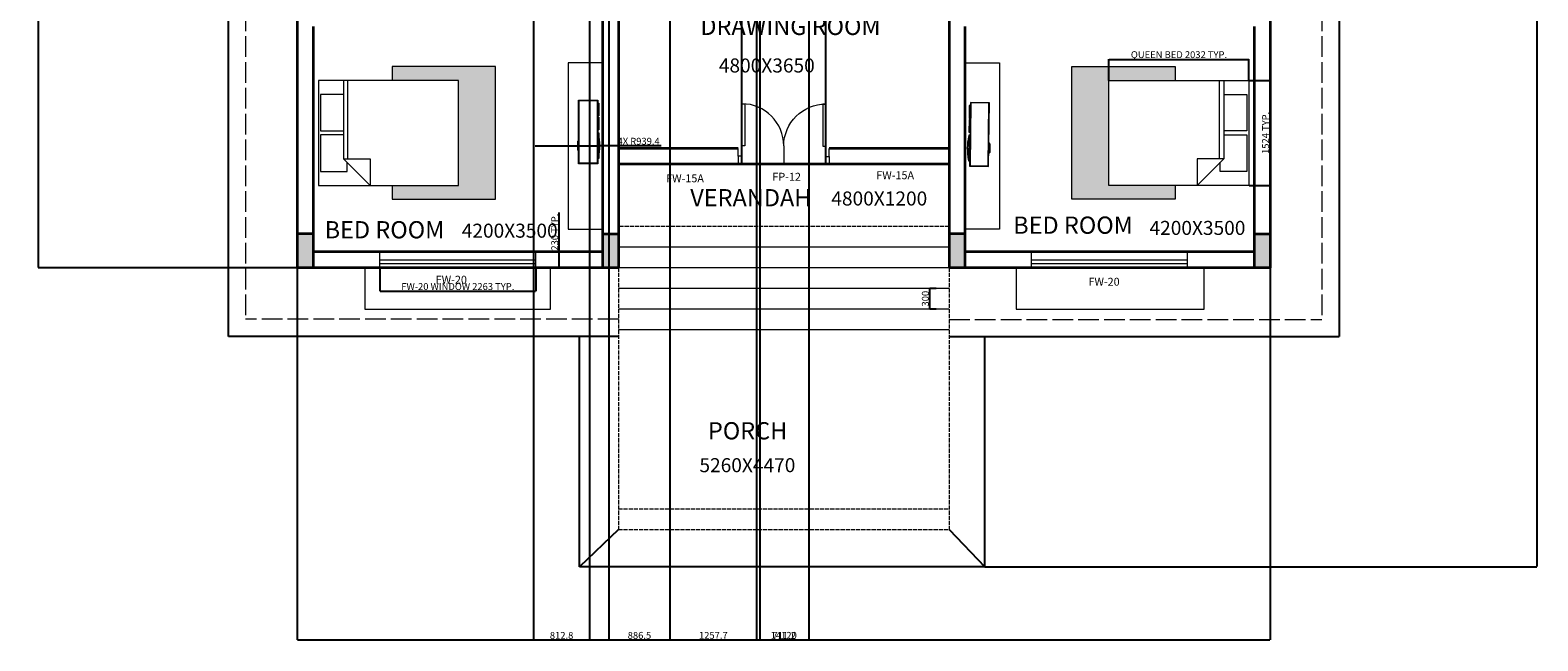
# Model space of a CAD drawing. Units: millimetres. Extents: x -17016 to 4866, y -18325 to 4338.
# Tile 1 of 5: x -17016 to 4866, y -18325 to -9462. Entities that reach past the tile are written whole.
import ezdxf

# ---------------------------------------------------------------- set-up
doc = ezdxf.new("R2010")
doc.units = ezdxf.units.MM
doc.header["$LTSCALE"] = 5
doc.linetypes.add('ACAD_ISO02W100', pattern=[15, 12, -3])
for name, color, linetype, lineweight in [('A-ANNO-DIMS', 2, 'Continuous', 18), ('A-ANNO-IDEN', 3, 'Continuous', 18), ('A-AREA-IDEN', 7, 'Continuous', 25), ('A-COLS', 7, 'Continuous', 35), ('A-COLS-PATT', 252, 'Continuous', 13), ('A-DOOR', 3, 'Continuous', 18), ('A-FLOR-OTLN', 8, 'Continuous', 25), ('A-FLOR-PATT', 252, 'Continuous', 13), ('A-FLOR-STRS', 7, 'Continuous', 18), ('A-FURN', 8, 'Continuous', 18), ('A-GLAZ', 4, 'Continuous', 18), ('A-ROOF', 8, 'Continuous', 18), ('A-ROOF-OVHD', 8, 'ACAD_ISO02W100', 13), ('A-WALL', 7, 'Continuous', 35)]:
    doc.layers.add(name, color=color, linetype=linetype, lineweight=lineweight)
doc.styles.get("Standard").update_dxf_attribs({"font": 'arial.ttf'})
doc.dimstyles.new('Copy of ISO-25', dxfattribs={"dimtxt": 100, "dimasz": 2.5, "dimexe": 1.25, "dimexo": 0.625, "dimtad": 1, "dimdec": 0, "dimtxsty": 'Standard', "dimcen": 2.5, "dimadec": 0, "dimazin": 0, "dimtfac": 1, "dimtdec": 0, "dimtmove": 0, "dimatfit": 3, "dimfxl": 1, "dimarcsym": 0})

# ---------------------------------------------------------------- blocks, each defined once
blk = doc.blocks.new('Bed - Queen')
for p, q in [((0, -80.00003), (0, 0)), ((0, 0), (59.99999, 0)), ((59.99999, 0), (59.99999, -80.00003)), ((7.99999, -1.2), (28.79998, -1.2)), ((7.99999, -14.4), (7.99999, -1.2)), ((28.79998, -1.2), (28.79998, -14.4)), ((31.19999, -1.2), (51.99999, -1.2)), ((31.19999, -14.4), (31.19999, -1.2)), ((51.99999, -1.2), (51.99999, -16.4)), ((0, -14.4), (44.8, -14.4)), ((44.8, -16.8), (0, -16.8)), ((59.99999, -29.6), (44.8, -14.4)), ((44.8, -14.4), (44.8, -29.6)), ((51.99999, -16.4), (46.79936, -16.4)), ((44.8, -29.6), (59.99999, -29.6)), ((59.99999, -80.00003), (0, -80.00003))]:
    blk.add_line(p, q)
blk = doc.blocks.new('Entertainment Center')
for p, q in [((-4, 0), (-5, -1)), ((4, 0), (-4, 0)), ((5, -1), (4, 0)), ((-17, -19), (-17, -1)), ((-17, -1), (43, -1)), ((-16.5, -18.5), (-16.5, -1.5)), ((-16.5, -1.5), (42.5, -1.5)), ((42.5, -1.5), (42.5, -18.5)), ((43, -1), (43, -19)), ((43, -19), (-17, -19)), ((42.5, -18.5), (-16.5, -18.5)), ((-12, -20), (-12, -19)), ((12, -20), (-12, -20)), ((12, -19), (12, -20)), ((15, -20), (15, -19)), ((27, -20), (15, -20)), ((27, -19), (27, -20)), ((28, -20), (28, -19)), ((40, -20), (28, -20)), ((40, -19), (40, -20))]:
    blk.add_line(p, q)
blk.add_arc((0, 40), 61, 259.6111, 280.3889)
blk = doc.blocks.new('*D15')
at = {"layer": 'A-ANNO-DIMS', "color": 0, "lineweight": -2, "ltscale": 5, "transparency": 16777216}
for p, q in [((-3867, -13209), (-3960, -13209)), ((-3959, -13507), (-3959, -13212)), ((-3867, -13509), (-3960, -13509))]:
    blk.add_line(p, q, dxfattribs=at)
at = {"layer": 'A-ANNO-DIMS', "color": 0, "ltscale": 5, "transparency": 16777216}
for points in [[(-3959, -13212), (-3958, -13212), (-3959, -13209)], [(-3959, -13507), (-3958, -13507), (-3959, -13509)]]:
    blk.add_solid(points, dxfattribs=at)
at = {"layer": 'Defpoints', "color": 0, "ltscale": 5, "transparency": 16777216}
for p in [(-3959, -13209), (-3867, -13209), (-3867, -13509)]:
    blk.add_point(p, dxfattribs=at)
at = {"layer": 'A-ANNO-DIMS', "color": 0, "ltscale": 5, "transparency": 16777216, "insert": (-4011, -13359), "char_height": 100, "attachment_point": 5, "rotation": 90}
blk.add_mtext('300', dxfattribs=at)
blk = doc.blocks.new('*U3')
for p, q in [((0, 0), (0, -6)), ((24, 0), (24, -6))]:
    blk.add_line(p, q)
blk.add_lwpolyline([(0, 0), (0, 24), (1.75, 24), (1.75, 0)], close=True)
blk.add_arc((0, 0), 24, 0, 90)
blk = doc.blocks.new('WIN-FW20')
for p, q in [((0, 0), (0, 230)), ((2263, 0), (2263, 230)), ((0, 115), (2263, 115)), ((0, 60), (2263, 60))]:
    blk.add_line(p, q)
blk = doc.blocks.new('*D24')
at = {"layer": 'A-ANNO-DIMS', "color": 0, "lineweight": -2, "ltscale": 5, "transparency": 16777216}
for p, q in [((-1359, -10190), (-1359, -9884)), ((-1356, -9886), (671, -9886)), ((673, -10190), (673, -9884))]:
    blk.add_line(p, q, dxfattribs=at)
at = {"layer": 'A-ANNO-DIMS', "color": 0, "ltscale": 5, "transparency": 16777216}
for points in [[(-1356, -9885), (-1356, -9886), (-1359, -9886)], [(671, -9885), (671, -9886), (673, -9886)]]:
    blk.add_solid(points, dxfattribs=at)
at = {"layer": 'Defpoints', "color": 0, "ltscale": 5, "transparency": 16777216}
for p in [(673, -9886), (-1359, -10191), (673, -10191)]:
    blk.add_point(p, dxfattribs=at)
at = {"layer": 'A-ANNO-DIMS', "color": 0, "ltscale": 5, "transparency": 16777216, "insert": (-343, -9830), "char_height": 100, "attachment_point": 5}
blk.add_mtext('QUEEN BED 2032 TYP.', dxfattribs=at)
blk = doc.blocks.new('*D25')
at = {"layer": 'A-ANNO-DIMS', "color": 0, "lineweight": -2, "ltscale": 5, "transparency": 16777216}
for p, q in [((674, -10191), (979, -10191)), ((978, -10193), (978, -11712)), ((674, -11715), (979, -11715))]:
    blk.add_line(p, q, dxfattribs=at)
at = {"layer": 'A-ANNO-DIMS', "color": 0, "ltscale": 5, "transparency": 16777216}
for points in [[(978, -10193), (979, -10193), (978, -10191)], [(978, -11712), (979, -11712), (978, -11715)]]:
    blk.add_solid(points, dxfattribs=at)
at = {"layer": 'Defpoints', "color": 0, "ltscale": 5, "transparency": 16777216}
for p in [(673, -10191), (673, -11715), (978, -11715)]:
    blk.add_point(p, dxfattribs=at)
at = {"layer": 'A-ANNO-DIMS', "color": 0, "ltscale": 5, "transparency": 16777216, "insert": (927, -10953), "char_height": 100, "attachment_point": 5, "rotation": 90}
blk.add_mtext('1524 TYP.', dxfattribs=at)
blk = doc.blocks.new('*D30')
at = {"layer": 'A-ANNO-DIMS', "color": 0, "lineweight": -2, "ltscale": 5, "transparency": 16777216}
for p, q in [((-11941, -12910), (-11941, -13250)), ((-9678, -12910), (-9678, -13250)), ((-11938, -13249), (-9680, -13249))]:
    blk.add_line(p, q, dxfattribs=at)
at = {"layer": 'A-ANNO-DIMS', "color": 0, "ltscale": 5, "transparency": 16777216}
for points in [[(-11938, -13248), (-11938, -13249), (-11941, -13249)], [(-9680, -13248), (-9680, -13249), (-9678, -13249)]]:
    blk.add_solid(points, dxfattribs=at)
at = {"layer": 'Defpoints', "color": 0, "ltscale": 5, "transparency": 16777216}
for p in [(-11941, -12909), (-9678, -12909), (-9678, -13249)]:
    blk.add_point(p, dxfattribs=at)
at = {"layer": 'A-ANNO-DIMS', "color": 0, "ltscale": 5, "transparency": 16777216, "insert": (-10809, -13196), "char_height": 100, "attachment_point": 5}
blk.add_mtext('FW-20 WINDOW 2263 TYP.', dxfattribs=at)
blk = doc.blocks.new('*D31')
at = {"layer": 'A-ANNO-DIMS', "color": 0, "lineweight": -2, "ltscale": 5, "transparency": 16777216}
for p, q in [((-9338, -12679), (-9338, -12109)), ((-9677, -12679), (-9337, -12679)), ((-9338, -12907), (-9338, -12682)), ((-9677, -12909), (-9337, -12909))]:
    blk.add_line(p, q, dxfattribs=at)
at = {"layer": 'A-ANNO-DIMS', "color": 0, "ltscale": 5, "transparency": 16777216}
for points in [[(-9338, -12682), (-9338, -12682), (-9338, -12679)], [(-9338, -12907), (-9338, -12907), (-9338, -12909)]]:
    blk.add_solid(points, dxfattribs=at)
at = {"layer": 'Defpoints', "color": 0, "ltscale": 5, "transparency": 16777216}
for p in [(-9678, -12679), (-9338, -12679), (-9678, -12909)]:
    blk.add_point(p, dxfattribs=at)
at = {"layer": 'A-ANNO-DIMS', "color": 0, "ltscale": 5, "transparency": 16777216, "insert": (-9390, -12393), "char_height": 100, "attachment_point": 5, "rotation": 90}
blk.add_mtext('230 TYP.', dxfattribs=at)
blk = doc.blocks.new('*D47')
at = {"layer": 'A-ANNO-DIMS', "color": 0, "lineweight": -2, "ltscale": 5, "transparency": 16777216}
for p, q in [((3524, 3161), (4853, 3161)), ((4852, 3158), (4852, -17248)), ((-3160, -17251), (4853, -17251))]:
    blk.add_line(p, q, dxfattribs=at)
at = {"layer": 'A-ANNO-DIMS', "color": 0, "ltscale": 5, "transparency": 16777216}
for points in [[(4851, 3158), (4852, 3158), (4852, 3161)], [(4851, -17248), (4852, -17248), (4852, -17251)]]:
    blk.add_solid(points, dxfattribs=at)
at = {"layer": 'Defpoints', "color": 0, "ltscale": 5, "transparency": 16777216}
for p in [(3524, 3161), (-3160, -17251), (4852, -17251)]:
    blk.add_point(p, dxfattribs=at)
at = {"layer": 'A-ANNO-DIMS', "color": 0, "ltscale": 5, "transparency": 16777216, "insert": (4800, -7045), "char_height": 100, "attachment_point": 5, "rotation": 90}
blk.add_mtext('20412', dxfattribs=at)
blk = doc.blocks.new('*D48')
at = {"layer": 'A-ANNO-DIMS', "color": 0, "lineweight": -2, "ltscale": 5, "transparency": 16777216}
for p, q in [((-13139, -12910), (-13139, -18312)), ((981, -12910), (981, -18312)), ((-13137, -18311), (978, -18311))]:
    blk.add_line(p, q, dxfattribs=at)
at = {"layer": 'A-ANNO-DIMS', "color": 0, "ltscale": 5, "transparency": 16777216}
for points in [[(-13137, -18310), (-13137, -18311), (-13139, -18311)], [(978, -18310), (978, -18311), (981, -18311)]]:
    blk.add_solid(points, dxfattribs=at)
at = {"layer": 'Defpoints', "color": 0, "ltscale": 5, "transparency": 16777216}
for p in [(-13139, -12909), (981, -12909), (981, -18311)]:
    blk.add_point(p, dxfattribs=at)
at = {"layer": 'A-ANNO-DIMS', "color": 0, "ltscale": 5, "transparency": 16777216, "insert": (-6079, -18259), "char_height": 100, "attachment_point": 5}
blk.add_mtext('14120', dxfattribs=at)
blk = doc.blocks.new('*D49')
at = {"layer": 'A-ANNO-DIMS', "color": 0, "lineweight": -2, "ltscale": 5, "transparency": 16777216}
for p, q in [((-14607, 2161), (-16900, 2161)), ((-16899, 2158), (-16899, -12907)), ((-13140, -12909), (-16900, -12909))]:
    blk.add_line(p, q, dxfattribs=at)
at = {"layer": 'A-ANNO-DIMS', "color": 0, "ltscale": 5, "transparency": 16777216}
for points in [[(-16899, 2158), (-16898, 2158), (-16899, 2161)], [(-16899, -12907), (-16898, -12907), (-16899, -12909)]]:
    blk.add_solid(points, dxfattribs=at)
at = {"layer": 'Defpoints', "color": 0, "ltscale": 5, "transparency": 16777216}
for p in [(-14606, 2161), (-16899, -12909), (-13139, -12909)]:
    blk.add_point(p, dxfattribs=at)
at = {"layer": 'A-ANNO-DIMS', "color": 0, "ltscale": 5, "transparency": 16777216, "insert": (-16950, -5374), "char_height": 100, "attachment_point": 5, "rotation": 90}
blk.add_mtext('15070', dxfattribs=at)
blk = doc.blocks.new('*D50')
at = {"layer": 'A-ANNO-DIMS', "color": 0, "lineweight": -2, "ltscale": 5, "transparency": 16777216}
for p, q in [((-9709, -2800), (-9709, -18312)), ((-8896, -2800), (-8896, -18312)), ((-9707, -18311), (-8899, -18311))]:
    blk.add_line(p, q, dxfattribs=at)
at = {"layer": 'A-ANNO-DIMS', "color": 0, "ltscale": 5, "transparency": 16777216}
for points in [[(-9707, -18310), (-9707, -18311), (-9709, -18311)], [(-8899, -18310), (-8899, -18311), (-8896, -18311)]]:
    blk.add_solid(points, dxfattribs=at)
at = {"layer": 'Defpoints', "color": 0, "ltscale": 5, "transparency": 16777216}
for p in [(-9709, -2799), (-8896, -2799), (-8896, -18311)]:
    blk.add_point(p, dxfattribs=at)
at = {"layer": 'A-ANNO-DIMS', "color": 0, "ltscale": 5, "transparency": 16777216, "insert": (-9303, -18259), "char_height": 100, "attachment_point": 5}
blk.add_mtext('812.8', dxfattribs=at)
blk = doc.blocks.new('*D51')
at = {"layer": 'A-ANNO-DIMS', "color": 0, "lineweight": -2, "ltscale": 5, "transparency": 16777216}
for p, q in [((-6428, -2800), (-6428, -18312)), ((-5716, -2800), (-5716, -18312)), ((-6425, -18311), (-5719, -18311))]:
    blk.add_line(p, q, dxfattribs=at)
at = {"layer": 'A-ANNO-DIMS', "color": 0, "ltscale": 5, "transparency": 16777216}
for points in [[(-6425, -18310), (-6425, -18311), (-6428, -18311)], [(-5719, -18310), (-5719, -18311), (-5716, -18311)]]:
    blk.add_solid(points, dxfattribs=at)
at = {"layer": 'Defpoints', "color": 0, "ltscale": 5, "transparency": 16777216}
for p in [(-6428, -2799), (-5716, -2799), (-5716, -18311)]:
    blk.add_point(p, dxfattribs=at)
at = {"layer": 'A-ANNO-DIMS', "color": 0, "ltscale": 5, "transparency": 16777216, "insert": (-6072, -18260), "char_height": 100, "attachment_point": 5}
blk.add_mtext('711.2', dxfattribs=at)
blk = doc.blocks.new('*D53')
at = {"layer": 'A-ANNO-DIMS', "color": 0, "lineweight": -2, "ltscale": 5, "transparency": 16777216}
for p, q in [((-6689, -11408), (-6689, 4222)), ((-6686, 4221), (-5472, 4221)), ((-5470, -11408), (-5470, 4222))]:
    blk.add_line(p, q, dxfattribs=at)
at = {"layer": 'A-ANNO-DIMS', "color": 0, "ltscale": 5, "transparency": 16777216}
for points in [[(-6686, 4221), (-6686, 4220), (-6689, 4221)], [(-5472, 4221), (-5472, 4220), (-5470, 4221)]]:
    blk.add_solid(points, dxfattribs=at)
at = {"layer": 'Defpoints', "color": 0, "ltscale": 5, "transparency": 16777216}
for p in [(-5470, 4221), (-6689, -11409), (-5470, -11409)]:
    blk.add_point(p, dxfattribs=at)
at = {"layer": 'A-ANNO-DIMS', "color": 0, "ltscale": 5, "transparency": 16777216, "insert": (-6079, 4272), "char_height": 100, "attachment_point": 5}
blk.add_mtext('1219.2', dxfattribs=at)
blk = doc.blocks.new('*D54')
at = {"layer": 'A-ANNO-DIMS', "color": 0, "lineweight": -2, "ltscale": 5, "transparency": 16777216}
for p, q in [((-7730, 1141), (-7730, -18312)), ((-6472, 1141), (-6472, -18312)), ((-7727, -18311), (-6475, -18311))]:
    blk.add_line(p, q, dxfattribs=at)
at = {"layer": 'A-ANNO-DIMS', "color": 0, "ltscale": 5, "transparency": 16777216}
for points in [[(-7727, -18310), (-7727, -18311), (-7730, -18311)], [(-6475, -18310), (-6475, -18311), (-6472, -18311)]]:
    blk.add_solid(points, dxfattribs=at)
at = {"layer": 'Defpoints', "color": 0, "ltscale": 5, "transparency": 16777216}
for p in [(-7730, 1141), (-6472, 1141), (-6472, -18311)]:
    blk.add_point(p, dxfattribs=at)
at = {"layer": 'A-ANNO-DIMS', "color": 0, "ltscale": 5, "transparency": 16777216, "insert": (-7101, -18259), "char_height": 100, "attachment_point": 5}
blk.add_mtext('1257.7', dxfattribs=at)
blk = doc.blocks.new('*D56')
at = {"layer": 'A-ANNO-DIMS', "color": 0, "lineweight": -2, "ltscale": 5, "transparency": 16777216}
for p, q in [((-8616, -2525), (-8616, -18312)), ((-7730, -2525), (-7730, -18312)), ((-8614, -18311), (-7732, -18311))]:
    blk.add_line(p, q, dxfattribs=at)
at = {"layer": 'A-ANNO-DIMS', "color": 0, "ltscale": 5, "transparency": 16777216}
for points in [[(-8614, -18310), (-8614, -18311), (-8616, -18311)], [(-7732, -18310), (-7732, -18311), (-7730, -18311)]]:
    blk.add_solid(points, dxfattribs=at)
at = {"layer": 'Defpoints', "color": 0, "ltscale": 5, "transparency": 16777216}
for p in [(-8616, -2525), (-7730, -2525), (-7730, -18311)]:
    blk.add_point(p, dxfattribs=at)
at = {"layer": 'A-ANNO-DIMS', "color": 0, "ltscale": 5, "transparency": 16777216, "insert": (-8173, -18259), "char_height": 100, "attachment_point": 5}
blk.add_mtext('886.5', dxfattribs=at)
blk = doc.blocks.new('*D61')
at = {"layer": 'A-ANNO-DIMS', "color": 0, "lineweight": -2, "ltscale": 5, "transparency": 16777216}
for p, q in [((-9688, -11139), (-8748, -11139)), ((-7858, -11139), (-8746, -11139))]:
    blk.add_line(p, q, dxfattribs=at)
at = {"layer": 'A-ANNO-DIMS', "color": 0, "ltscale": 5, "transparency": 16777216}
blk.add_solid([(-8746, -11138), (-8746, -11139), (-8748, -11139)], dxfattribs=at)
at = {"layer": 'Defpoints', "color": 0, "ltscale": 5, "transparency": 16777216}
for p in [(-9688, -11139), (-8748, -11139)]:
    blk.add_point(p, dxfattribs=at)
at = {"layer": 'A-ANNO-DIMS', "color": 0, "ltscale": 5, "transparency": 16777216, "insert": (-8185, -11087), "char_height": 100, "attachment_point": 5, "rotation": 0}
blk.add_mtext('4X R939.4', dxfattribs=at)

msp = doc.modelspace()

# ---------------------------------------------------------------- hatches: boundary and pattern name
at = {"layer": 'A-COLS-PATT', "ltscale": 5}
h = msp.add_hatch(color=256, dxfattribs=at)
h.dxf.hatch_style = 1
h.paths.add_polyline_path([(980.82, -12419.11), (750.82, -12419.11), (750.82, -12909.11), (980.82, -12909.11)])
h.paths.add_polyline_path([(-3449.18, -12419.11), (-3679.18, -12419.11), (-3679.18, -12909.11), (-3449.18, -12909.11)])
h.paths.add_polyline_path([(-8479.18, -12419.11), (-8709.18, -12419.11), (-8709.18, -12909.11), (-8479.18, -12909.11)])
h.paths.add_polyline_path([(-12909.18, -12419.11), (-13139.18, -12419.11), (-13139.18, -12909.11), (-12909.18, -12909.11)])
at = {"layer": 'A-FLOR-PATT'}
h = msp.add_hatch(dxfattribs=at)
h.set_pattern_fill('ANSI38', color=256, scale=25)
h.set_pattern_definition([(45, (-20162.07, -7174.37), (-56.1266, 56.1266), []), (135, (-20162.07, -7174.37), (-168.3798, 56.1266), [198.4375, -119.0625])])
h.paths.add_polyline_path([(-1358.58, -10190.51), (-396.23, -10190.51), (-396.23, -9990.51), (-1896.23, -9990.51), (-1896.23, -11914.51), (-396.23, -11914.51), (-396.23, -11714.51), (-1358.58, -11714.51)])
h.paths.add_polyline_path([(-10262.12, -9990.51), (-11762.12, -9990.51), (-11762.12, -10190.51), (-10799.77, -10190.51), (-10799.77, -11714.51), (-11762.12, -11714.51), (-11762.12, -11914.51), (-10262.12, -11914.51)])
h.paths.add_polyline_path([(-9722.08, 912.47), (-11222.08, 912.47), (-11222.08, 712.47), (-10260.08, 712.47), (-10260.08, -811.53), (-11222.08, -811.53), (-11222.08, -1011.53), (-9722.08, -1011.53)])
h.paths.add_polyline_path([(-2814.18, 912.47), (-4314.18, 912.47), (-4314.18, 712.47), (-3352.18, 712.47), (-3352.18, -811.53), (-4314.18, -811.53), (-4314.18, -1011.53), (-2814.18, -1011.53)])

# ---------------------------------------------------------------- linework, layer by layer
at = {"layer": 'A-COLS', "ltscale": 5}
for p, q in [((-12909.18, -12419.11), (-13139.18, -12419.11)), ((-8712.53, -12419.11), (-8479.18, -12419.11)), ((-3449.18, -12419.11), (-3679.18, -12419.11)), ((750.82, -12419.11), (980.82, -12419.11))]:
    msp.add_line(p, q, dxfattribs=at)
at = {"layer": 'A-DOOR', "ltscale": 5}
for p, q in [((-6738.77, -11292.35), (-6738.77, -11179.11)), ((-6688.77, -11292.35), (-6738.77, -11292.35)), ((-6738.77, -11292.35), (-6738.77, -11409.11)), ((-6688.77, -11292.35), (-6688.77, -11409.11)), ((-6079.18, -11179.11), (-6079.18, -11409.11)), ((-5469.58, -11295.88), (-5419.58, -11295.88)), ((-5469.58, -11295.88), (-5469.58, -11409.11)), ((-5419.58, -11295.88), (-5419.58, -11179.11)), ((-5419.58, -11295.88), (-5419.58, -11409.11))]:
    msp.add_line(p, q, dxfattribs=at)
at = {"layer": 'A-FLOR-OTLN', "ltscale": 5}
for p, q in [((-14139.18, -13909.11), (-14139.18, -3799.11)), ((1980.82, -3799.11), (1980.82, -13909.11)), ((-8479.18, -13909.11), (-14139.18, -13909.11)), ((-9045.18, -17250.83), (-9045.18, -13909.11)), ((-3679.18, -13909.11), (1980.82, -13909.11)), ((-3160.48, -17250.83), (-3160.48, -13909.11)), ((-8479.18, -16709.11), (-9045.18, -17250.83)), ((-3679.18, -16709.11), (-3160.48, -17250.83)), ((-3160.48, -17250.83), (-9045.18, -17250.83))]:
    msp.add_line(p, q, dxfattribs=at)
at = {"layer": 'A-FLOR-PATT'}
for points in [[(-11762.12, -11714.51), (-11762.12, -11914.51), (-10262.12, -11914.51), (-10262.12, -9990.51), (-11762.12, -9990.51), (-11762.12, -10190.51)], [(-396.23, -11714.51), (-396.23, -11914.51), (-1896.23, -11914.51), (-1896.23, -9990.51), (-396.23, -9990.51), (-396.23, -10190.51)]]:
    msp.add_lwpolyline(points, dxfattribs=at)
at = {"layer": 'A-FLOR-STRS'}
for p, q in [((-3679.18, -12609.11), (-8479.18, -12609.11)), ((-3679.18, -12909.11), (-8479.18, -12909.11)), ((-3679.18, -12909.11), (-8479.18, -12909.11)), ((-3679.18, -13209.11), (-8479.18, -13209.11)), ((-3679.18, -13509.11), (-8479.18, -13509.11)), ((-3679.18, -13809.11), (-8479.18, -13809.11))]:
    msp.add_line(p, q, dxfattribs=at)
at = {"layer": 'A-FURN'}
for points in [[(-8709.18, -9935.79), (-9209.18, -9935.79), (-9209.18, -12350.21), (-8709.18, -12350.21)], [(-3449.18, -9935.79), (-2949.18, -9935.79), (-2949.18, -12350.21), (-3449.18, -12350.21)]]:
    msp.add_lwpolyline(points, dxfattribs=at)
at = {"layer": 'A-ROOF', "ltscale": 5}
for p, q in [((-12158.58, -12909.11), (-12158.58, -13509.11)), ((-9462.93, -13509.11), (-9462.93, -12909.11)), ((-2706.33, -12909.11), (-2706.33, -13509.11)), ((22.86, -13509.11), (22.86, -12909.11)), ((-12158.58, -13509.11), (-9462.93, -13509.11)), ((-2706.33, -13509.11), (22.86, -13509.11))]:
    msp.add_line(p, q, dxfattribs=at)
at = {"layer": 'A-ROOF-OVHD', "ltscale": 5}
for p, q in [((-13889.18, -7299.11), (-13889.18, -13655.43)), ((1730.82, -7299.11), (1730.82, -13659.11)), ((-8479.18, -13655.43), (-13889.18, -13655.43)), ((-3679.18, -13659.11), (1730.82, -13659.11))]:
    msp.add_line(p, q, dxfattribs=at)
at = {"layer": 'A-ROOF-OVHD'}
for p, q in [((-3679.18, -12309.11), (-8479.18, -12309.11)), ((-8479.18, -12909.11), (-8479.18, -16709.11)), ((-3679.18, -12909.11), (-3679.18, -16709.11)), ((-8479.18, -16409.11), (-3679.18, -16409.11)), ((-8479.18, -16709.11), (-3679.18, -16709.11))]:
    msp.add_line(p, q, dxfattribs=at)
at = {"layer": 'A-WALL'}
for p, q in [((980.82, -7299.11), (980.82, -12909.11)), ((-13139.18, -7529.11), (-13139.18, -12909.11)), ((-8709.18, -7529.11), (-8709.18, -12909.11)), ((-8479.18, -7529.11), (-8479.18, -12909.11)), ((-3679.18, -7529.11), (-3679.18, -12909.11)), ((-12909.18, -9409.11), (-12909.18, -12909.11)), ((-3449.18, -9409.11), (-3449.18, -12909.11)), ((750.82, -9409.11), (750.82, -12909.11)), ((-6738.77, -11179.11), (-8479.18, -11179.11)), ((-6078.84, -11179.11), (-6079.18, -11179.11)), ((-3679.18, -11179.11), (-5419.58, -11179.11)), ((-6688.77, -11409.11), (-8479.18, -11409.11)), ((-3679.18, -11409.11), (-6688.77, -11409.11)), ((-8709.18, -12679.11), (-12909.18, -12679.11)), ((750.82, -12679.11), (-3449.18, -12679.11)), ((-8479.18, -12909.11), (-13139.18, -12909.11)), ((980.82, -12909.11), (-3679.18, -12909.11))]:
    msp.add_line(p, q, dxfattribs=at)

# ---------------------------------------------------------------- block references
at = {"layer": 'A-DOOR', "rotation": 359.8339641169521}
for p, xscale, yscale, zscale in [((-6688.33, -11139.95), 25.40000000000001, 25.40000000000001, 25.40000000000001), ((-5469.14, -11143.48), -25.40000000000001, 25.4, 25.4)]:
    msp.add_blockref('*U3', p, dxfattribs=dict(at, xscale=xscale, yscale=yscale, zscale=zscale))
at = {"layer": 'A-FURN', "extrusion": (-1e-16, 0, -1), "xscale": 25.4, "yscale": 25.4, "zscale": 25.4, "rotation": 269.9999999999998}
msp.add_blockref('Bed - Queen', (12831.77, -10190.51), dxfattribs=at)
at = {"layer": 'A-FURN', "extrusion": (1e-16, 0, -1), "xscale": -25.4, "yscale": 25.4, "zscale": 25.4, "rotation": 90.00000000000024}
msp.add_blockref('Bed - Queen', (-673.42, -10190.51), dxfattribs=at)
at = {"layer": 'A-FURN', "yscale": 15.40069445834287, "zscale": 15.40069445834287}
for p, xscale, rotation in [((-9071.63, -11138.83), 15.40069445834287, 89.99999999999999), ((-3086.46, -11176.69), -15.40069445834287, 269.2751324688127)]:
    msp.add_blockref('Entertainment Center', p, dxfattribs=dict(at, xscale=xscale, rotation=rotation))
at = {"layer": 'A-GLAZ'}
for p in [(-11940.79, -12909.11), (-2480.79, -12909.11)]:
    msp.add_blockref('WIN-FW20', p, dxfattribs=at)

# ---------------------------------------------------------------- texts
at = {"layer": 'A-ANNO-IDEN', "ltscale": 5}
for s, p in [('FW-15A', (-7785.17, -11669.25)), ('FP-12', (-6243.42, -11647.15)), ('FW-15A', (-4735.35, -11625.08)), ('FW-20', (-11129.65, -13141.37)), ('FW-20', (-1656.08, -13170.81))]:
    msp.add_text(s, height=114.837, dxfattribs=at).set_placement(p)
at = {"layer": 'A-AREA-IDEN', "ltscale": 5}
for s, height, p in [('DRAWING ROOM', 250, (-7289.61, -9531.88)), ('4800X3650', 203.546, (-7020.82, -10076.32)), ('VERANDAH', 250, (-7435.43, -12018.53)), ('4800X1200', 203.546, (-5388.19, -12006.71)), ('BED ROOM', 250, (-12741.85, -12483.63)), ('BED ROOM', 250, (-2748.55, -12417.12)), ('4200X3500', 203.546, (-770.54, -12433.64)), ('4200X3500', 203.546, (-10752.14, -12473.96)), ('PORCH', 250, (-7179.19, -15401.41)), ('5260X4470', 203.546, (-7302.52, -15877.52))]:
    msp.add_text(s, height=height, dxfattribs=at).set_placement(p)

# ---------------------------------------------------------------- dimensions: what is measured, and where the dimension line sits
at = {"layer": 'A-ANNO-DIMS', "ltscale": 5}
for base, p1, p2, override, picture, middle in [((-5469.58, 4220.64), (-6688.77, -11409.11), (-5469.58, -11409.11), {"dimdec": 1, "dimlfac": 1, "dimrnd": 0, "dimzin": 0, "dimdsep": 46, "dimlunit": 2}, '*D53', (-6079.18, 4272.32)), ((-6472.15, -18310.58), (-7729.85, 1141.22), (-6472.15, 1141.22), {"dimdec": 1, "dimlfac": 1, "dimrnd": 0, "dimzin": 0, "dimdsep": 46, "dimlunit": 2}, '*D54', (-7101, -18258.9)), ((-7729.85, -18310.58), (-8616.38, -2524.75), (-7729.85, -2524.75), {"dimdec": 1, "dimlfac": 1, "dimrnd": 0, "dimzin": 0, "dimdsep": 46, "dimlunit": 2}, '*D56', (-8173.11, -18258.9)), ((-8896.38, -18310.58), (-9709.18, -2799.11), (-8896.38, -2799.11), {"dimdec": 1, "dimlfac": 1, "dimrnd": 0, "dimzin": 0, "dimdsep": 46, "dimlunit": 2}, '*D50', (-9302.78, -18258.9)), ((-5716.38, -18310.58), (-6427.58, -2799.11), (-5716.38, -2799.11), {"dimdec": 1, "dimlfac": 1, "dimrnd": 0, "dimzin": 0, "dimdsep": 46, "dimlunit": 2}, '*D51', (-6071.98, -18259.75)), ((980.82, -18310.58), (-13139.18, -12909.11), (980.82, -12909.11), {"dimdec": 0, "dimlfac": 1, "dimrnd": 0, "dimzin": 0, "dimdsep": 46, "dimlunit": 2}, '*D48', (-6079.18, -18258.9))]:
    dim = msp.add_linear_dim(base=base, p1=p1, p2=p2, dimstyle='Copy of ISO-25', override=override, dxfattribs=at)
    dim.commit()
    dim.dimension.update_dxf_attribs({"geometry": picture, "text_midpoint": middle})
for base, p1, p2, override, picture, middle in [((4851.91, -17250.83), (3523.62, 3160.89), (-3160.48, -17250.83), {"dimdec": 0, "dimlfac": 1, "dimrnd": 0, "dimzin": 0, "dimdsep": 46, "dimlunit": 2}, '*D47', (4800.22, -7044.97)), ((-16898.81, -12909.11), (-14606.38, 2160.89), (-13139.18, -12909.11), {"dimdec": 0, "dimlfac": 1, "dimrnd": 0, "dimzin": 0, "dimdsep": 46, "dimlunit": 2}, '*D49', (-16950.49, -5374.11)), ((-3958.88, -13209.11), (-3866.68, -13509.11), (-3866.68, -13209.11), {"dimclrd": 0, "dimclre": 0, "dimclrt": 0}, '*D15', (-4010.59, -13359.11))]:
    dim = msp.add_linear_dim(base=base, p1=p1, p2=p2, angle=90, dimstyle='Copy of ISO-25', override=override, dxfattribs=at)
    dim.commit()
    dim.dimension.update_dxf_attribs({"geometry": picture, "text_midpoint": middle})
for base, p1, p2, text, picture, middle in [((673.42, -9885.71), (-1358.58, -10190.51), (673.42, -10190.51), 'QUEEN BED <> TYP.', '*D24', (-342.58, -9830.31)), ((-9677.57, -13248.6), (-11940.79, -12909.11), (-9677.57, -12909.11), 'FW-20 WINDOW <> TYP.', '*D30', (-10809.18, -13196.2))]:
    dim = msp.add_linear_dim(base=base, p1=p1, p2=p2, text=text, dimstyle='Copy of ISO-25', override={"dimdec": 0, "dimlfac": 1, "dimrnd": 0, "dimzin": 0, "dimdsep": 46, "dimlunit": 2}, dxfattribs=at)
    dim.commit()
    dim.dimension.update_dxf_attribs({"geometry": picture, "text_midpoint": middle})
for base, p1, p2, angle, picture, middle in [((978.22, -11714.51), (673.42, -10190.51), (673.42, -11714.51), 270, '*D25', (926.53, -10952.51)), ((-9338.08, -12679.11), (-9677.57, -12909.11), (-9677.57, -12679.11), 90, '*D31', (-9389.8, -12392.91))]:
    dim = msp.add_linear_dim(base=base, p1=p1, p2=p2, angle=angle, text='<> TYP.', dimstyle='Copy of ISO-25', override={"dimdec": 0, "dimlfac": 1, "dimrnd": 0, "dimzin": 0, "dimdsep": 46, "dimlunit": 2}, dxfattribs=at)
    dim.commit()
    dim.dimension.update_dxf_attribs({"geometry": picture, "text_midpoint": middle})
dim = msp.add_radius_dim(center=(-9687.65, -11138.83), mpoint=(-8748.21, -11138.83), text='4X <>', dimstyle='Copy of ISO-25', override={"dimdec": 1, "dimlfac": 1, "dimrnd": 0, "dimzin": 0, "dimdsep": 46, "dimlunit": 2}, dxfattribs=at)
dim.commit()
dim.dimension.update_dxf_attribs({"geometry": '*D61', "text_midpoint": (-8184.55, -11138.82), "dimtype": 164})

doc.saveas('drawing.dxf')
